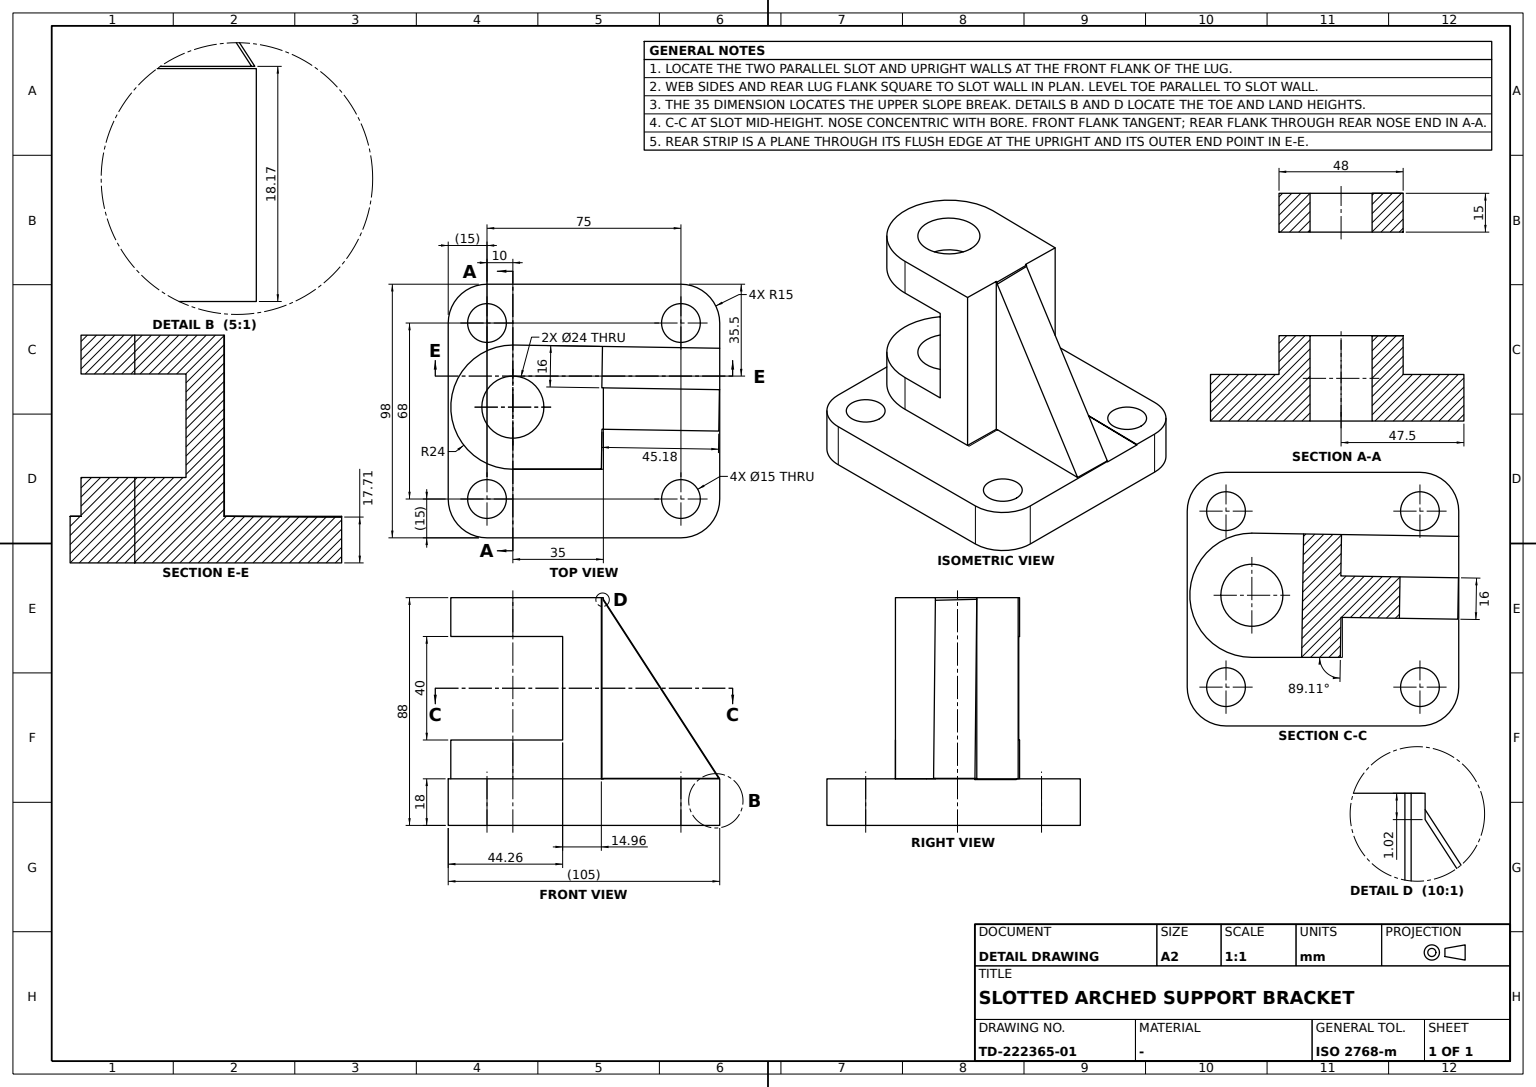
CATIA V5 part; units mm, degrees
sketch "Sketch1" plane through (0, 0, 0) normal (0, 0, 1) x (0, 1, 0)
  line L0 (0, 0) -> (98, 0)
  line L1 (98, 0) -> (98, -105)
  line L2 (98, -105) -> (0, -105)
  line L3 (0, -105) -> (0, 0)
  dimension "length L1" = 105
  dimension "length L2" = 98
  constraint horizontal L0 x-axis
  constraint horizontal L2 x-axis
  constraint vertical L1 y-axis
  constraint vertical L3 y-axis
extrude "Pad1" add sketch "Sketch1" along normal blind 18
fillet "Fillet1" radius 15 4 edges at (105, 0, 9) (105, 98, 9) (0, 98, 9) (0, 0, 9)
sketch "Sketch2" plane through (96.3517, 13.2807, 18) normal (0, 0, 1) x (1, 0, 0)
  point P0 (-6.3517, 1.7193)
  arc A0 (-6.3517, -13.2807) -> (8.6483, 1.7193) centre (-6.3517, 1.7193) ccw construction
  constraint concentricity A0 P0
hole "Hole1" at (90, 15, 18) direction (0, 0, -1) diameter 15 end up to next
sketch "Sketch3" plane through (14.3226, 6.1676, 18) normal (0, 0, 1) x (1, 0, 0)
  point P0 (0.6774, 8.8324)
  arc A0 (-14.3226, 8.8324) -> (0.6774, -6.1676) centre (0.6774, 8.8324) ccw construction
  constraint concentricity A0 P0
hole "Hole2" at (15, 15, 18) direction (0, 0, -1) diameter 15 end up to next
sketch "Sketch4" plane through (94.0199, 81.2916, 18) normal (0, 0, 1) x (1, 0, 0)
  point P0 (-4.0199, 1.7084)
  arc A0 (10.9801, 1.7084) -> (-4.0199, 16.7084) centre (-4.0199, 1.7084) ccw construction
  constraint concentricity A0 P0
hole "Hole3" at (90, 83, 18) direction (0, 0, -1) diameter 15 end up to next
sketch "Sketch5" plane through (15.2811, 84.8728, 18) normal (0, 0, 1) x (1, 0, 0)
  point P0 (-0.2811, -1.8728)
  arc A0 (-0.2811, 13.1272) -> (-15.2811, -1.8728) centre (-0.2811, -1.8728) ccw construction
  constraint concentricity A0 P0
hole "Hole4" at (15, 83, 18) direction (0, 0, -1) diameter 15 end up to next
sketch "Sketch6" plane through (0, 0, 18) normal (0, 0, 1) x (0, 1, 0)
  arc A0 (74.5, -25) -> (26.5, -25) centre (50.5, -25) ccw
  point P0 (50.5, -25)
  line L0 (26.5, -25) -> (26.5, -60)
  line L1 (74.5, -25) -> (73.9535, -60)
  line L2 (26.5, -60) -> (73.9535, -60)
  line L3 (98, -105) -> (98, 0) construction
  line L4 (0, -105) -> (98, -105) construction
  dimension "radius A0" = 24
  dimension "length L0" = 35
  dimension "distance P0 L3" = 47.5
  dimension "distance L2 L4" = 45
  constraint tangency L0 A0
  constraint horizontal L2 x-axis
extrude "Pad2" add sketch "Sketch6" along normal blind 70
sketch "Sketch7" plane through (15.6575, 49.8322, 88) normal (0, 0, 1) x (1, 0, 0)
  point P0 (9.3425, 0.6678)
  arc A0 (9.3425, 24.6678) -> (9.3425, -23.3322) centre (9.3425, 0.6678) ccw construction
  constraint concentricity A0 P0
hole "Hole5" at (25, 50.5, 88) direction (0, 0, -1) diameter 24 end up to next
sketch "Sketch8" plane through (1.169, 74.8721, 0) normal (0.0156, 0.9999, 0) x (-0.9999, 0.0156, 0)
  line L0 (-43.8382, 73) -> (1.1618, 73)
  line L1 (1.1618, 73) -> (1.1618, 33)
  line L2 (1.1618, 33) -> (-43.8382, 33)
  line L3 (-43.8382, 33) -> (-43.8382, 73)
  line L4 (-58.8382, 18) -> (-58.8382, 88) construction
  dimension "length L0" = 45
  dimension "length L1" = 40
  dimension "distance L3 L4" = 15
  constraint horizontal L0 x-axis
  constraint horizontal L2 x-axis
  constraint vertical L1 y-axis
  constraint vertical L3 y-axis
extrude "Pocket1" cut sketch "Sketch8" against normal up to next
sketch "Sketch9" plane through (1.169, 74.8721, 0) normal (0.0156, 0.9999, 0) x (-0.9999, 0.0156, 0)
  line L0 (-58.8382, 87.7511) -> (-58.8382, 18.1718)
  line L1 (-58.8382, 18.1718) -> (-103.9782, 18.1718)
  line L2 (-103.9782, 18.1718) -> (-58.8382, 87.7511)
  constraint vertical L0 y-axis
  constraint horizontal L1 x-axis
extrude "Pad3" add sketch "Sketch9" against normal blind 48
sketch "Sketch10" plane through (1.169, 74.8721, 0) normal (0.0156, 0.9999, 0) x (-0.9999, 0.0156, 0)
  line L0 (-105.7512, 17.7026) -> (-58.4968, 90.0758)
  line L1 (-58.4968, 90.0758) -> (-58.4968, 18.0008)
  line L2 (-58.4968, 18.0008) -> (-105.7512, 17.7026)
  constraint vertical L1 y-axis
extrude "Pocket2" cut sketch "Sketch10" against normal blind 16
sketch "Sketch11" plane through (0.4197, 26.878, 0) normal (-0.0156, -0.9999, 0) x (0.9999, -0.0156, 0)
  line L0 (58.7971, 18.0304) -> (58.7971, 89.8526)
  line L1 (58.7971, 89.8526) -> (104.8514, 18.0304)
  line L2 (104.8514, 18.0304) -> (58.7971, 18.0304)
  constraint vertical L0 y-axis
  constraint horizontal L2 x-axis
extrude "Pocket3" cut sketch "Sketch11" against normal blind 16
properties part number "catia 19"
